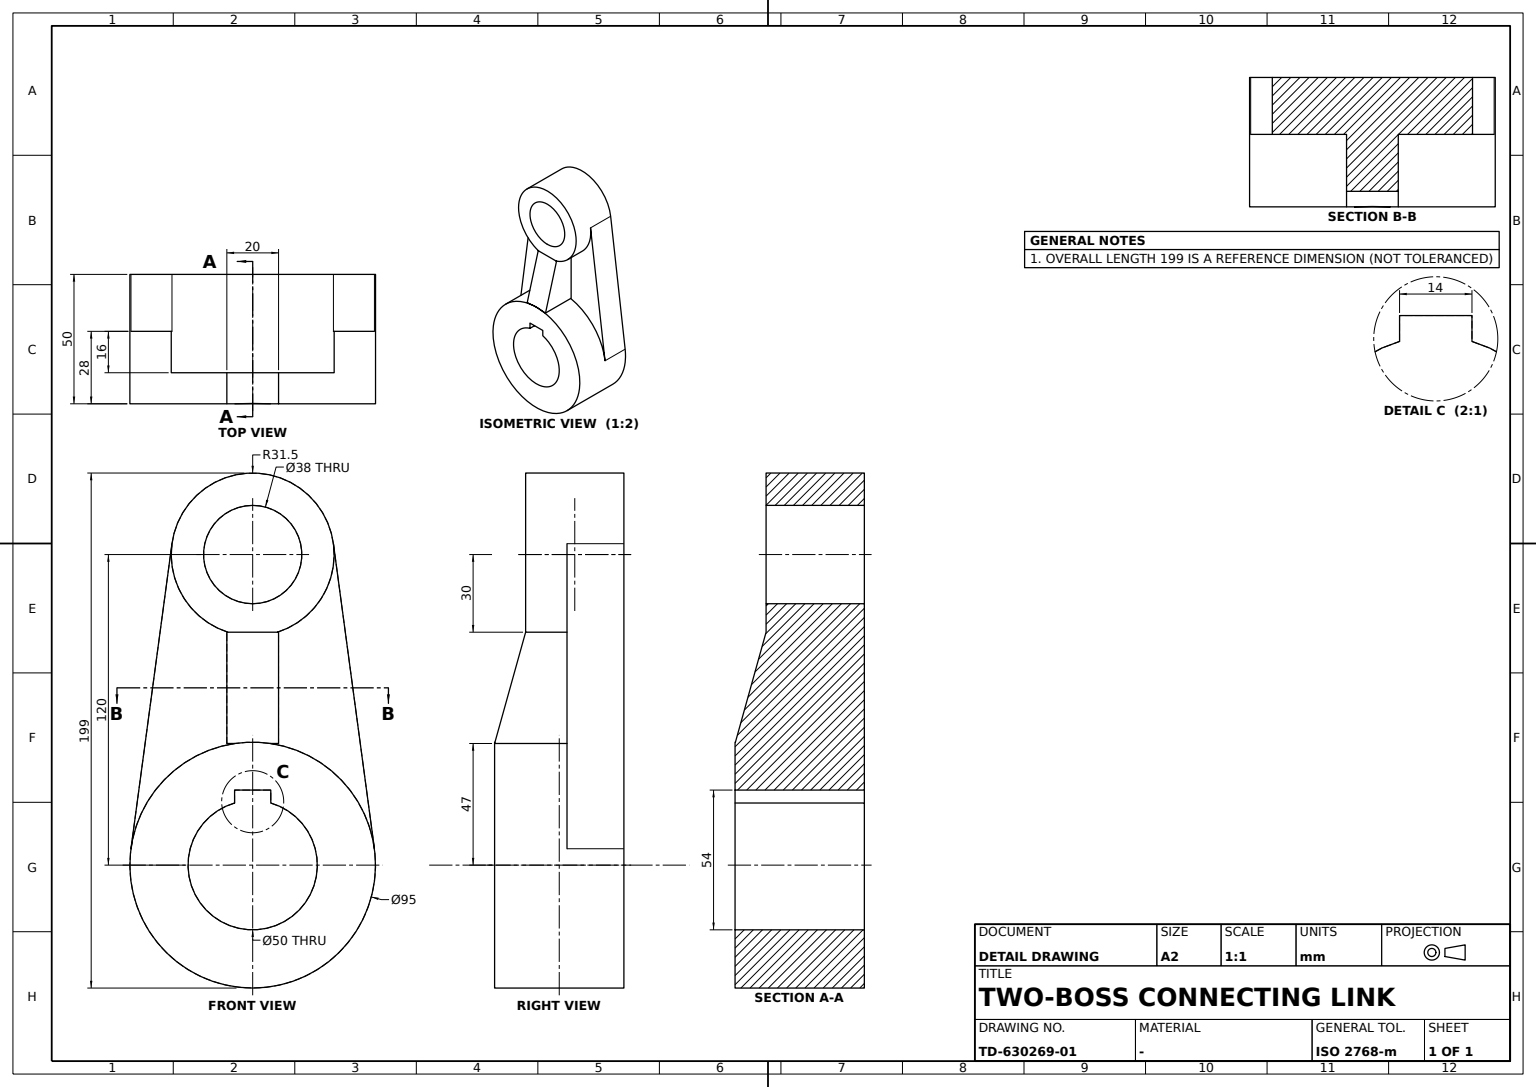
CATIA V5 part; units mm, degrees
sketch "Sketch1" plane through (0, 0, 0) normal (1, 0, 0) x (0, 1, 0)
  circle A0 centre (0, 0) radius 47.5
  arc A1 (-7, 24) -> (7, 24) centre (0, 0) ccw
  line L0 (-7, 24) -> (-7, 29)
  line L1 (-7, 29) -> (7, 29)
  line L2 (7, 29) -> (7, 24)
  dimension "radius A0" = 47.5
  dimension "radius A1" = 25
  dimension "length L2" = 5
  dimension "length L1" = 14
  constraint vertical L0 y-axis
  constraint vertical L2 y-axis
  constraint horizontal L1 x-axis
  constraint symmetry L0 L2 y-axis
extrude "Pad1" add sketch "Sketch1" along normal mid plane 50
sketch "Sketch2" plane through (-25, 0, 0) normal (-1, 0, 0) x (0, -1, 0)
  arc A0 (31.2187, 124.2) -> (-31.2187, 124.2) centre (0, 120) ccw
  point P0 (0, 120)
  point P1 (-47.0759, 6.3333)
  line L0 (-47.0759, 6.3333) -> (-31.2187, 124.2)
  line L1 (31.2187, 124.2) -> (47.0759, 6.3333)
  point P2 (47.0759, 6.3333)
  circle A1 centre (0, 0) radius 47.5 construction
  circle A2 centre (0, 0) radius 47.5 construction
  circle A3 centre (0, 0) radius 47.5 construction
  circle A4 centre (0, 0) radius 47.5 construction
  arc A5 (47.0759, 6.3333) -> (-47.0759, 6.3333) centre (0, 0) ccw
  dimension "radius A0" = 31.5
  dimension "distance P0 origin" = 120
  constraint coincidence P0 y-axis
  constraint coincidence P2 A1
  constraint coincidence P1 A2
  constraint tangency L0 A3
  constraint tangency L1 A4
  constraint tangency L0 A0
  constraint tangency L1 A0
extrude "Pad2" add sketch "Sketch2" against normal blind 22
sketch "Sketch3" plane through (-3, 0, 0) normal (1, 0, 0) x (0, 1, 0)
  circle A0 centre (0, 120) radius 31.5
  point P0 (0, 120)
  point P1 (0, 88.5)
  circle A1 centre (0, 120) radius 19
  point P2 (0, 101)
  arc A2 (31.2187, 124.2) -> (-31.2187, 124.2) centre (0, 120) ccw construction
  dimension "radius A0" = 31.5
  dimension "radius A1" = 19
  constraint coincidence P0 y-axis
  constraint coincidence A0 P1
  constraint coincidence P1 y-axis
  constraint coincidence A1 P2
  constraint coincidence P2 y-axis
  constraint concentricity A0 A2
  constraint concentricity A1 A0
extrude "Pad3" add sketch "Sketch3" along normal blind 16
sketch "Pocket1 profile" plane through (-3, 0, 0) normal (1, 0, 0) x (0, 1, 0)
  circle A0 centre (0, 120) radius 19
extrude "Pocket1" cut sketch "Pocket1 profile" against normal up to next
sketch "Sketch4" plane through (0, 0, 0) normal (0, 1, 0) x (-1, 0, 0)
  line L0 (-13, 90) -> (-25, 47)
  line L1 (-25, 47) -> (3, 47)
  line L2 (3, 47) -> (3, 90)
  line L3 (3, 90) -> (-13, 90)
  line L4 (3, 124.2) -> (3, 6.3333) construction
  dimension "D1" = 47
  dimension "D2" = 30
  dimension "length L3" = 16
  dimension "length L1" = 28
  constraint horizontal L1 x-axis
  constraint horizontal L3 x-axis
  constraint coincidence L4 L2
extrude "Pad4" add sketch "Sketch4" along normal mid plane 20
